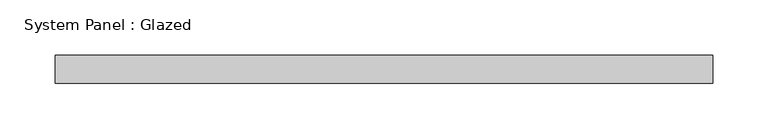
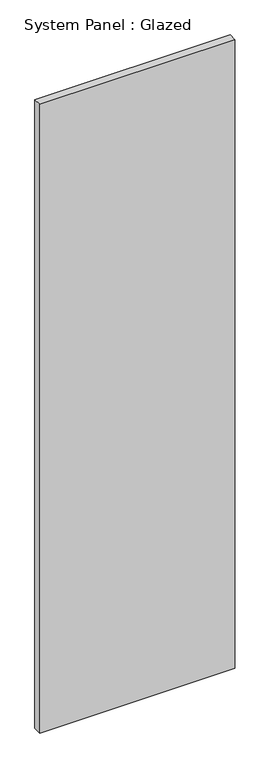
"""IFC4 building model written with IfcOpenShell, lengths in millimetres: plate geometry, System Panel : Glazed."""

from ifc_helpers import new_model, si_unit, origin, origin_with_axes, place, context, project, spatial, polyline, outline, extrude, source, transform, mapped, element, save


def system_panel_glazed_4c4e158e(model_context):
    return source(origin(), model_context, "Body", "SweptSolid", [
        extrude(outline(polyline([(298.45, 19.05), (-298.45, 19.05), (-298.45, 44.45), (298.45, 44.45), (298.45, 19.05)])), origin_with_axes(), (0.0, 0.0, 1.0), 2032.0),
    ])


if __name__ == "__main__":
    model = new_model("IFC4")
    model_context = context("Model", 3, world=origin())
    ifc_project = project(units=[si_unit("LENGTHUNIT", "METRE", prefix="MILLI")], contexts=[model_context])
    site = spatial("IfcSite", under=ifc_project)
    building = spatial("IfcBuilding", under=site)
    placement = place(None, origin())
    system_panel_glazed_shape = system_panel_glazed_4c4e158e(model_context)
    element("IfcPlate", 1, ObjectType="System Panel : Glazed", at=placement, inside=building, context=model_context, shape_type="MappedRepresentation", body=[
        mapped(system_panel_glazed_shape, transform((0.0, 0.0, 0.0), x_axis=(1.0, 0.0, 0.0), y_axis=(0.0, 1.0, 0.0), z_axis=(0.0, 0.0, 1.0))),
    ])
    save(model, "model.ifc")

# Revit data of these elements
# Type "System Panel : Glazed"
#   Construction Type Id = "GSP4R"
#   Analytic Construction = "1/8 in Pilkington single glazing"
#   Visual Light Transmittance = 0.9
#   Solar Heat Gain Coefficient = 0.86
#   Heat Transfer Coefficient (U) = 1.18115 BTU/(h·ft²·°F)
#   Define Thermal Properties by = 1
# Element 1 (IfcPlate, "System Panel : Glazed")
#   Materials on its faces: "Glass"
# Materials
#   "Glass": class "Glass", colour RGB 0 128 192, transparency 0.75, Description = "Soda Lime Glass", Cost = 0
